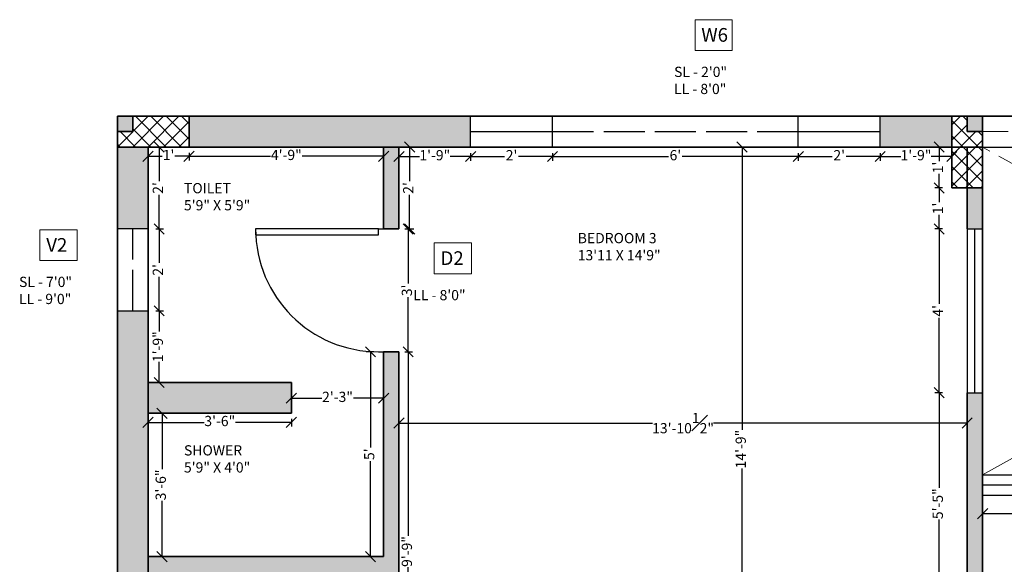
# Model space of a CAD drawing. Units: inches. Extents: x 1365 to 2091, y 1589 to 2091.
# Tile 4 of 8: x 1365 to 1654, y 1932 to 2091. Entities that reach past the tile are written whole.
import ezdxf

# ---------------------------------------------------------------- set-up
doc = ezdxf.new("R2010")
doc.units = ezdxf.units.IN
doc.linetypes.add('ACAD_ISO02W100', pattern=[15, 12, -3])
for name, color, linetype, lineweight in [('A-ANNO-DIMS', 2, 'Continuous', 18), ('A-ANNO-SYMB', 12, 'Continuous', 18), ('A-AREA-IDEN', 7, 'Continuous', 18), ('A-COLS', 7, 'Continuous', 35), ('A-COLS-MARK-PATT', 114, 'Continuous', 13), ('A-COLS-PATT', 1, 'Continuous', 13), ('A-DOOR', 4, 'Continuous', 25), ('A-FLOR-HRAL', 7, 'Continuous', 25), ('A-FLOR-OPEN', 7, 'Continuous', 25), ('A-FLOR-OPEN-HIDN', 1, 'ACAD_ISO02W100', 18), ('A-GLAZ', 150, 'Continuous', 30), ('A-GLAZ-HIDN', 150, 'ACAD_ISO02W100', 30), ('A-WALL', 7, 'Continuous', 35), ('A-WALL-PATT', 253, 'Continuous', 13)]:
    doc.layers.add(name, color=color, linetype=linetype, lineweight=lineweight)
doc.styles.get("Standard").update_dxf_attribs({"font": 'arial.ttf'})
doc.dimstyles.new('ISO-25', dxfattribs={"dimtxt": 3, "dimasz": 3, "dimexe": 1.25, "dimexo": 0.625, "dimtad": 0, "dimlunit": 4, "dimtxsty": 'Standard', "dimblk": 'OBLIQUE', "dimcen": 2.5, "dimclrd": 254, "dimclre": 254, "dimclrt": 1, "dimadec": 0, "dimazin": 0, "dimtfac": 1, "dimtmove": 0, "dimatfit": 3, "dimfxl": 1, "dimfxlon": 1, "dimfrac": 1, "dimarcsym": 0})

# ---------------------------------------------------------------- blocks, each defined once
blk = doc.blocks.new('*U3')
for p, q in [((-36, 0), (-36, -6)), ((0, 0), (0, -6))]:
    blk.add_line(p, q)
blk.add_lwpolyline([(0, 0), (0, 36), (-1.75, 36), (-1.75, 0)], close=True)
blk.add_arc((0, 0), 36, 90, 180)
blk = doc.blocks.new('_Oblique')
at = {"color": 0, "linetype": 'ByBlock', "lineweight": -2}
blk.add_line((-0.5, -0.5), (0.5, 0.5), dxfattribs=at)
blk = doc.blocks.new('*D8')
at = {"layer": 'A-ANNO-DIMS', "color": 0, "lineweight": -2, "transparency": 16777216}
for p, q in [((1402.75, 2052.14), (1402.75, 2049.89)), ((1414.75, 2052.14), (1414.75, 2049.89)), ((1402.75, 2051.14), (1406.89, 2051.14)), ((1414.75, 2051.14), (1410.62, 2051.14))]:
    blk.add_line(p, q, dxfattribs=at)
at = {"layer": 'Defpoints', "color": 0, "transparency": 16777216}
for p in [(1402.75, 2053.86), (1414.75, 2053.86), (1414.75, 2051.14)]:
    blk.add_point(p, dxfattribs=at)
at = {"layer": 'A-ANNO-DIMS', "color": 0, "lineweight": -2, "transparency": 16777216, "xscale": 3, "yscale": 3, "zscale": 3, "rotation": 180}
blk.add_blockref('_Oblique', (1402.75, 2051.14), dxfattribs=at)
at = {"layer": 'A-ANNO-DIMS', "color": 0, "lineweight": -2, "transparency": 16777216, "xscale": 3, "yscale": 3, "zscale": 3}
blk.add_blockref('_Oblique', (1414.75, 2051.14), dxfattribs=at)
at = {"layer": 'A-ANNO-DIMS', "color": 0, "transparency": 16777216, "insert": (1408.75, 2051.14), "char_height": 3, "attachment_point": 5}
blk.add_mtext("1'", dxfattribs=at)
blk = doc.blocks.new('*D9')
at = {"layer": 'A-ANNO-DIMS', "color": 0, "lineweight": -2, "transparency": 16777216}
for p, q in [((1414.75, 2052.14), (1414.75, 2049.89)), ((1471.75, 2052.14), (1471.75, 2049.89)), ((1414.75, 2051.14), (1438.58, 2051.14)), ((1471.75, 2051.14), (1447.93, 2051.14))]:
    blk.add_line(p, q, dxfattribs=at)
at = {"layer": 'Defpoints', "color": 0, "transparency": 16777216}
for p in [(1414.75, 2053.86), (1471.75, 2053.86), (1471.75, 2051.14)]:
    blk.add_point(p, dxfattribs=at)
at = {"layer": 'A-ANNO-DIMS', "color": 0, "lineweight": -2, "transparency": 16777216, "xscale": 3, "yscale": 3, "zscale": 3, "rotation": 180}
blk.add_blockref('_Oblique', (1414.75, 2051.14), dxfattribs=at)
at = {"layer": 'A-ANNO-DIMS', "color": 0, "lineweight": -2, "transparency": 16777216, "xscale": 3, "yscale": 3, "zscale": 3}
blk.add_blockref('_Oblique', (1471.75, 2051.14), dxfattribs=at)
at = {"layer": 'A-ANNO-DIMS', "color": 0, "transparency": 16777216, "insert": (1443.25, 2051.14), "char_height": 3, "attachment_point": 5}
blk.add_mtext('4\'-9"', dxfattribs=at)
blk = doc.blocks.new('*D10')
at = {"layer": 'A-ANNO-DIMS', "color": 0, "lineweight": -2, "transparency": 16777216}
for p, q in [((1476.25, 2052.07), (1476.25, 2049.82)), ((1497.25, 2052.07), (1497.25, 2049.82)), ((1476.25, 2051.07), (1482.28, 2051.07)), ((1497.25, 2051.07), (1491.22, 2051.07))]:
    blk.add_line(p, q, dxfattribs=at)
at = {"layer": 'Defpoints', "color": 0, "transparency": 16777216}
for p in [(1476.25, 2053.86), (1497.25, 2053.86), (1476.25, 2051.07)]:
    blk.add_point(p, dxfattribs=at)
at = {"layer": 'A-ANNO-DIMS', "color": 0, "lineweight": -2, "transparency": 16777216, "xscale": 3, "yscale": 3, "zscale": 3, "rotation": 180}
blk.add_blockref('_Oblique', (1476.25, 2051.07), dxfattribs=at)
at = {"layer": 'A-ANNO-DIMS', "color": 0, "lineweight": -2, "transparency": 16777216, "xscale": 3, "yscale": 3, "zscale": 3}
blk.add_blockref('_Oblique', (1497.25, 2051.07), dxfattribs=at)
at = {"layer": 'A-ANNO-DIMS', "color": 0, "transparency": 16777216, "insert": (1486.75, 2051.07), "char_height": 3, "attachment_point": 5}
blk.add_mtext('1\'-9"', dxfattribs=at)
blk = doc.blocks.new('*D11')
at = {"layer": 'A-ANNO-DIMS', "color": 0, "lineweight": -2, "transparency": 16777216}
for p, q in [((1497.25, 2052.07), (1497.25, 2049.82)), ((1521.25, 2052.07), (1521.25, 2049.82)), ((1497.25, 2051.07), (1507.22, 2051.07)), ((1521.25, 2051.07), (1511.28, 2051.07))]:
    blk.add_line(p, q, dxfattribs=at)
at = {"layer": 'Defpoints', "color": 0, "transparency": 16777216}
for p in [(1497.25, 2053.86), (1521.25, 2053.86), (1521.25, 2051.07)]:
    blk.add_point(p, dxfattribs=at)
at = {"layer": 'A-ANNO-DIMS', "color": 0, "lineweight": -2, "transparency": 16777216, "xscale": 3, "yscale": 3, "zscale": 3, "rotation": 180}
blk.add_blockref('_Oblique', (1497.25, 2051.07), dxfattribs=at)
at = {"layer": 'A-ANNO-DIMS', "color": 0, "lineweight": -2, "transparency": 16777216, "xscale": 3, "yscale": 3, "zscale": 3}
blk.add_blockref('_Oblique', (1521.25, 2051.07), dxfattribs=at)
at = {"layer": 'A-ANNO-DIMS', "color": 0, "transparency": 16777216, "insert": (1509.25, 2051.07), "char_height": 3, "attachment_point": 5}
blk.add_mtext("2'", dxfattribs=at)
blk = doc.blocks.new('*D12')
at = {"layer": 'A-ANNO-DIMS', "color": 0, "lineweight": -2, "transparency": 16777216}
for p, q in [((1521.25, 2052.07), (1521.25, 2049.82)), ((1593.25, 2052.07), (1593.25, 2049.82)), ((1521.25, 2051.07), (1555.24, 2051.07)), ((1593.25, 2051.07), (1559.27, 2051.07))]:
    blk.add_line(p, q, dxfattribs=at)
at = {"layer": 'Defpoints', "color": 0, "transparency": 16777216}
for p in [(1521.25, 2053.86), (1593.25, 2053.86), (1593.25, 2051.07)]:
    blk.add_point(p, dxfattribs=at)
at = {"layer": 'A-ANNO-DIMS', "color": 0, "lineweight": -2, "transparency": 16777216, "xscale": 3, "yscale": 3, "zscale": 3, "rotation": 180}
blk.add_blockref('_Oblique', (1521.25, 2051.07), dxfattribs=at)
at = {"layer": 'A-ANNO-DIMS', "color": 0, "lineweight": -2, "transparency": 16777216, "xscale": 3, "yscale": 3, "zscale": 3}
blk.add_blockref('_Oblique', (1593.25, 2051.07), dxfattribs=at)
at = {"layer": 'A-ANNO-DIMS', "color": 0, "transparency": 16777216, "insert": (1557.25, 2051.07), "char_height": 3, "attachment_point": 5}
blk.add_mtext("6'", dxfattribs=at)
blk = doc.blocks.new('*D13')
at = {"layer": 'A-ANNO-DIMS', "color": 0, "lineweight": -2, "transparency": 16777216}
for p, q in [((1593.25, 2052.07), (1593.25, 2049.82)), ((1617.25, 2052.07), (1617.25, 2049.82)), ((1593.25, 2051.07), (1603.22, 2051.07)), ((1617.25, 2051.07), (1607.28, 2051.07))]:
    blk.add_line(p, q, dxfattribs=at)
at = {"layer": 'Defpoints', "color": 0, "transparency": 16777216}
for p in [(1593.25, 2053.86), (1617.25, 2053.86), (1617.25, 2051.07)]:
    blk.add_point(p, dxfattribs=at)
at = {"layer": 'A-ANNO-DIMS', "color": 0, "lineweight": -2, "transparency": 16777216, "xscale": 3, "yscale": 3, "zscale": 3, "rotation": 180}
blk.add_blockref('_Oblique', (1593.25, 2051.07), dxfattribs=at)
at = {"layer": 'A-ANNO-DIMS', "color": 0, "lineweight": -2, "transparency": 16777216, "xscale": 3, "yscale": 3, "zscale": 3}
blk.add_blockref('_Oblique', (1617.25, 2051.07), dxfattribs=at)
at = {"layer": 'A-ANNO-DIMS', "color": 0, "transparency": 16777216, "insert": (1605.25, 2051.07), "char_height": 3, "attachment_point": 5}
blk.add_mtext("2'", dxfattribs=at)
blk = doc.blocks.new('*D14')
at = {"layer": 'A-ANNO-DIMS', "color": 0, "lineweight": -2, "transparency": 16777216}
for p, q in [((1617.25, 2052.07), (1617.25, 2049.82)), ((1638.25, 2052.07), (1638.25, 2049.82)), ((1617.25, 2051.07), (1623.28, 2051.07)), ((1638.25, 2051.07), (1632.22, 2051.07))]:
    blk.add_line(p, q, dxfattribs=at)
at = {"layer": 'Defpoints', "color": 0, "transparency": 16777216}
for p in [(1617.25, 2053.86), (1638.25, 2053.86), (1638.25, 2051.07)]:
    blk.add_point(p, dxfattribs=at)
at = {"layer": 'A-ANNO-DIMS', "color": 0, "lineweight": -2, "transparency": 16777216, "xscale": 3, "yscale": 3, "zscale": 3, "rotation": 180}
blk.add_blockref('_Oblique', (1617.25, 2051.07), dxfattribs=at)
at = {"layer": 'A-ANNO-DIMS', "color": 0, "lineweight": -2, "transparency": 16777216, "xscale": 3, "yscale": 3, "zscale": 3}
blk.add_blockref('_Oblique', (1638.25, 2051.07), dxfattribs=at)
at = {"layer": 'A-ANNO-DIMS', "color": 0, "transparency": 16777216, "insert": (1627.75, 2051.07), "char_height": 3, "attachment_point": 5}
blk.add_mtext('1\'-9"', dxfattribs=at)
blk = doc.blocks.new('*D16')
at = {"layer": 'A-ANNO-DIMS', "color": 0, "lineweight": -2, "transparency": 16777216}
for p, q in [((1404.99, 2053.86), (1407.24, 2053.86)), ((1405.99, 2053.86), (1405.99, 2043.89)), ((1405.99, 2029.86), (1405.99, 2039.83)), ((1404.99, 2029.86), (1407.24, 2029.86))]:
    blk.add_line(p, q, dxfattribs=at)
at = {"layer": 'Defpoints', "color": 0, "transparency": 16777216}
for p in [(1402.75, 2053.86), (1402.75, 2029.86), (1405.99, 2029.86)]:
    blk.add_point(p, dxfattribs=at)
at = {"layer": 'A-ANNO-DIMS', "color": 0, "lineweight": -2, "transparency": 16777216, "xscale": 3, "yscale": 3, "zscale": 3}
for p, rotation in [((1405.99, 2053.86), 90), ((1405.99, 2029.86), 270)]:
    blk.add_blockref('_Oblique', p, dxfattribs=dict(at, rotation=rotation))
at = {"layer": 'A-ANNO-DIMS', "color": 0, "transparency": 16777216, "insert": (1405.99, 2041.86), "char_height": 3, "attachment_point": 5, "rotation": 90}
blk.add_mtext("2'", dxfattribs=at)
blk = doc.blocks.new('*D17')
at = {"layer": 'A-ANNO-DIMS', "color": 0, "lineweight": -2, "transparency": 16777216}
for p, q in [((1404.99, 2029.86), (1407.24, 2029.86)), ((1405.99, 2029.86), (1405.99, 2019.89)), ((1405.99, 2005.86), (1405.99, 2015.83)), ((1404.99, 2005.86), (1407.24, 2005.86))]:
    blk.add_line(p, q, dxfattribs=at)
at = {"layer": 'Defpoints', "color": 0, "transparency": 16777216}
for p in [(1402.75, 2029.86), (1402.75, 2005.86), (1405.99, 2005.86)]:
    blk.add_point(p, dxfattribs=at)
at = {"layer": 'A-ANNO-DIMS', "color": 0, "lineweight": -2, "transparency": 16777216, "xscale": 3, "yscale": 3, "zscale": 3}
for p, rotation in [((1405.99, 2029.86), 90), ((1405.99, 2005.86), 270)]:
    blk.add_blockref('_Oblique', p, dxfattribs=dict(at, rotation=rotation))
at = {"layer": 'A-ANNO-DIMS', "color": 0, "transparency": 16777216, "insert": (1405.99, 2017.86), "char_height": 3, "attachment_point": 5, "rotation": 90}
blk.add_mtext("2'", dxfattribs=at)
blk = doc.blocks.new('*D18')
at = {"layer": 'A-ANNO-DIMS', "color": 0, "lineweight": -2, "transparency": 16777216}
for p, q in [((1404.99, 2005.86), (1407.24, 2005.86)), ((1405.99, 2005.86), (1405.99, 1999.83)), ((1405.99, 1984.86), (1405.99, 1990.89)), ((1404.99, 1984.86), (1407.24, 1984.86))]:
    blk.add_line(p, q, dxfattribs=at)
at = {"layer": 'Defpoints', "color": 0, "transparency": 16777216}
for p in [(1402.75, 2005.86), (1402.75, 1984.86), (1405.99, 1984.86)]:
    blk.add_point(p, dxfattribs=at)
at = {"layer": 'A-ANNO-DIMS', "color": 0, "lineweight": -2, "transparency": 16777216, "xscale": 3, "yscale": 3, "zscale": 3}
for p, rotation in [((1405.99, 2005.86), 90), ((1405.99, 1984.86), 270)]:
    blk.add_blockref('_Oblique', p, dxfattribs=dict(at, rotation=rotation))
at = {"layer": 'A-ANNO-DIMS', "color": 0, "transparency": 16777216, "insert": (1405.99, 1995.36), "char_height": 3, "attachment_point": 5, "rotation": 90}
blk.add_mtext('1\'-9"', dxfattribs=at)
blk = doc.blocks.new('*D19')
at = {"layer": 'A-ANNO-DIMS', "color": 0, "lineweight": -2, "transparency": 16777216}
for p, q in [((1444.75, 1979.27), (1444.75, 1981.52)), ((1444.75, 1980.27), (1453.62, 1980.27)), ((1471.75, 1980.27), (1462.89, 1980.27)), ((1471.75, 1979.27), (1471.75, 1981.52))]:
    blk.add_line(p, q, dxfattribs=at)
at = {"layer": 'Defpoints', "color": 0, "transparency": 16777216}
for p in [(1471.75, 1980.27), (1444.75, 1975.86), (1471.75, 1975.86)]:
    blk.add_point(p, dxfattribs=at)
at = {"layer": 'A-ANNO-DIMS', "color": 0, "lineweight": -2, "transparency": 16777216, "xscale": 3, "yscale": 3, "zscale": 3, "rotation": 180}
blk.add_blockref('_Oblique', (1444.75, 1980.27), dxfattribs=at)
at = {"layer": 'A-ANNO-DIMS', "color": 0, "lineweight": -2, "transparency": 16777216, "xscale": 3, "yscale": 3, "zscale": 3}
blk.add_blockref('_Oblique', (1471.75, 1980.27), dxfattribs=at)
at = {"layer": 'A-ANNO-DIMS', "color": 0, "transparency": 16777216, "insert": (1458.25, 1980.27), "char_height": 3, "attachment_point": 5}
blk.add_mtext('2\'-3"', dxfattribs=at)
blk = doc.blocks.new('*D20')
at = {"layer": 'A-ANNO-DIMS', "color": 0, "lineweight": -2, "transparency": 16777216}
for p, q in [((1402.75, 1974.2), (1402.75, 1971.95)), ((1444.75, 1974.2), (1444.75, 1971.95)), ((1402.75, 1973.2), (1419.14, 1973.2)), ((1444.75, 1973.2), (1428.37, 1973.2))]:
    blk.add_line(p, q, dxfattribs=at)
at = {"layer": 'Defpoints', "color": 0, "transparency": 16777216}
for p in [(1402.75, 1975.86), (1444.75, 1975.86), (1444.75, 1973.2)]:
    blk.add_point(p, dxfattribs=at)
at = {"layer": 'A-ANNO-DIMS', "color": 0, "lineweight": -2, "transparency": 16777216, "xscale": 3, "yscale": 3, "zscale": 3, "rotation": 180}
blk.add_blockref('_Oblique', (1402.75, 1973.2), dxfattribs=at)
at = {"layer": 'A-ANNO-DIMS', "color": 0, "lineweight": -2, "transparency": 16777216, "xscale": 3, "yscale": 3, "zscale": 3}
blk.add_blockref('_Oblique', (1444.75, 1973.2), dxfattribs=at)
at = {"layer": 'A-ANNO-DIMS', "color": 0, "transparency": 16777216, "insert": (1423.75, 1973.2), "char_height": 3, "attachment_point": 5}
blk.add_mtext('3\'-6"', dxfattribs=at)
blk = doc.blocks.new('*D21')
at = {"layer": 'A-ANNO-DIMS', "color": 0, "lineweight": -2, "transparency": 16777216}
for p, q in [((1405.84, 1975.86), (1408.09, 1975.86)), ((1406.84, 1975.86), (1406.84, 1959.47)), ((1406.84, 1933.86), (1406.84, 1950.25)), ((1405.84, 1933.86), (1408.09, 1933.86))]:
    blk.add_line(p, q, dxfattribs=at)
at = {"layer": 'Defpoints', "color": 0, "transparency": 16777216}
for p in [(1402.75, 1975.86), (1406.84, 1975.86), (1402.75, 1933.86)]:
    blk.add_point(p, dxfattribs=at)
at = {"layer": 'A-ANNO-DIMS', "color": 0, "lineweight": -2, "transparency": 16777216, "xscale": 3, "yscale": 3, "zscale": 3}
for p, rotation in [((1406.84, 1975.86), 90), ((1406.84, 1933.86), 270)]:
    blk.add_blockref('_Oblique', p, dxfattribs=dict(at, rotation=rotation))
at = {"layer": 'A-ANNO-DIMS', "color": 0, "transparency": 16777216, "insert": (1406.84, 1954.86), "char_height": 3, "attachment_point": 5, "rotation": 90}
blk.add_mtext('3\'-6"', dxfattribs=at)
blk = doc.blocks.new('*D22')
at = {"layer": 'A-ANNO-DIMS', "color": 0, "lineweight": -2, "transparency": 16777216}
for p, q in [((1468.92, 1993.86), (1466.67, 1993.86)), ((1467.92, 1993.86), (1467.92, 1965.86)), ((1467.92, 1933.86), (1467.92, 1961.85)), ((1468.92, 1933.86), (1466.67, 1933.86))]:
    blk.add_line(p, q, dxfattribs=at)
at = {"layer": 'Defpoints', "color": 0, "transparency": 16777216}
for p in [(1471.75, 1993.86), (1467.92, 1933.86), (1471.75, 1933.86)]:
    blk.add_point(p, dxfattribs=at)
at = {"layer": 'A-ANNO-DIMS', "color": 0, "lineweight": -2, "transparency": 16777216, "xscale": 3, "yscale": 3, "zscale": 3}
for p, rotation in [((1467.92, 1993.86), 90), ((1467.92, 1933.86), 270)]:
    blk.add_blockref('_Oblique', p, dxfattribs=dict(at, rotation=rotation))
at = {"layer": 'A-ANNO-DIMS', "color": 0, "transparency": 16777216, "insert": (1467.92, 1963.86), "char_height": 3, "attachment_point": 5, "rotation": 90}
blk.add_mtext("5'", dxfattribs=at)
blk = doc.blocks.new('*D93')
at = {"layer": 'A-ANNO-DIMS', "color": 0, "lineweight": -2, "transparency": 16777216}
for p, q in [((1647.25, 1947.47), (1647.25, 1945.22)), ((1819.75, 1947.47), (1819.75, 1945.22)), ((1647.25, 1946.47), (1725.72, 1946.47)), ((1819.75, 1946.47), (1741.29, 1946.47))]:
    blk.add_line(p, q, dxfattribs=at)
at = {"layer": 'Defpoints', "color": 0, "transparency": 16777216}
for p in [(1647.25, 1951.86), (1819.75, 1951.86), (1819.75, 1946.47)]:
    blk.add_point(p, dxfattribs=at)
at = {"layer": 'A-ANNO-DIMS', "color": 0, "lineweight": -2, "transparency": 16777216, "xscale": 3, "yscale": 3, "zscale": 3, "rotation": 180}
blk.add_blockref('_Oblique', (1647.25, 1946.47), dxfattribs=at)
at = {"layer": 'A-ANNO-DIMS', "color": 0, "lineweight": -2, "transparency": 16777216, "xscale": 3, "yscale": 3, "zscale": 3}
blk.add_blockref('_Oblique', (1819.75, 1946.47), dxfattribs=at)
at = {"layer": 'A-ANNO-DIMS', "color": 0, "transparency": 16777216, "insert": (1733.5, 1946.47), "char_height": 3, "attachment_point": 5}
blk.add_mtext('14\'-4{\\H1x;\\S1#2;}"', dxfattribs=at)
blk = doc.blocks.new('*D94')
at = {"layer": 'A-ANNO-DIMS', "color": 0, "lineweight": -2, "transparency": 16777216}
for p, q in [((1635.53, 2053.86), (1633.28, 2053.86)), ((1634.53, 2053.86), (1634.53, 2049.72)), ((1634.53, 2041.86), (1634.53, 2045.99)), ((1635.53, 2041.86), (1633.28, 2041.86))]:
    blk.add_line(p, q, dxfattribs=at)
at = {"layer": 'Defpoints', "color": 0, "transparency": 16777216}
for p in [(1638.25, 2053.86), (1634.53, 2041.86), (1638.25, 2041.86)]:
    blk.add_point(p, dxfattribs=at)
at = {"layer": 'A-ANNO-DIMS', "color": 0, "lineweight": -2, "transparency": 16777216, "xscale": 3, "yscale": 3, "zscale": 3}
for p, rotation in [((1634.53, 2053.86), 90), ((1634.53, 2041.86), 270)]:
    blk.add_blockref('_Oblique', p, dxfattribs=dict(at, rotation=rotation))
at = {"layer": 'A-ANNO-DIMS', "color": 0, "transparency": 16777216, "insert": (1634.53, 2047.86), "char_height": 3, "attachment_point": 5, "rotation": 90}
blk.add_mtext("1'", dxfattribs=at)
blk = doc.blocks.new('*D95')
at = {"layer": 'A-ANNO-DIMS', "color": 0, "lineweight": -2, "transparency": 16777216}
for p, q in [((1635.53, 2041.86), (1633.28, 2041.86)), ((1634.53, 2041.86), (1634.53, 2037.72)), ((1634.53, 2029.86), (1634.53, 2033.99)), ((1635.53, 2029.86), (1633.28, 2029.86))]:
    blk.add_line(p, q, dxfattribs=at)
at = {"layer": 'Defpoints', "color": 0, "transparency": 16777216}
for p in [(1638.25, 2041.86), (1634.53, 2029.86), (1642.75, 2029.86)]:
    blk.add_point(p, dxfattribs=at)
at = {"layer": 'A-ANNO-DIMS', "color": 0, "lineweight": -2, "transparency": 16777216, "xscale": 3, "yscale": 3, "zscale": 3}
for p, rotation in [((1634.53, 2041.86), 90), ((1634.53, 2029.86), 270)]:
    blk.add_blockref('_Oblique', p, dxfattribs=dict(at, rotation=rotation))
at = {"layer": 'A-ANNO-DIMS', "color": 0, "transparency": 16777216, "insert": (1634.53, 2035.86), "char_height": 3, "attachment_point": 5, "rotation": 90}
blk.add_mtext("1'", dxfattribs=at)
blk = doc.blocks.new('*D96')
at = {"layer": 'A-ANNO-DIMS', "color": 0, "lineweight": -2, "transparency": 16777216}
for p, q in [((1635.53, 2029.86), (1633.28, 2029.86)), ((1634.53, 2029.86), (1634.53, 2007.92)), ((1634.53, 1981.86), (1634.53, 2003.79)), ((1635.53, 1981.86), (1633.28, 1981.86))]:
    blk.add_line(p, q, dxfattribs=at)
at = {"layer": 'Defpoints', "color": 0, "transparency": 16777216}
for p in [(1642.75, 2029.86), (1634.53, 1981.86), (1642.75, 1981.86)]:
    blk.add_point(p, dxfattribs=at)
at = {"layer": 'A-ANNO-DIMS', "color": 0, "lineweight": -2, "transparency": 16777216, "xscale": 3, "yscale": 3, "zscale": 3}
for p, rotation in [((1634.53, 2029.86), 90), ((1634.53, 1981.86), 270)]:
    blk.add_blockref('_Oblique', p, dxfattribs=dict(at, rotation=rotation))
at = {"layer": 'A-ANNO-DIMS', "color": 0, "transparency": 16777216, "insert": (1634.53, 2005.86), "char_height": 3, "attachment_point": 5, "rotation": 90}
blk.add_mtext("4'", dxfattribs=at)
blk = doc.blocks.new('*D97')
at = {"layer": 'A-ANNO-DIMS', "color": 0, "lineweight": -2, "transparency": 16777216}
for p, q in [((1635.53, 1981.86), (1633.28, 1981.86)), ((1634.53, 1981.86), (1634.53, 1953.97)), ((1634.53, 1916.86), (1634.53, 1944.75)), ((1635.53, 1916.86), (1633.28, 1916.86))]:
    blk.add_line(p, q, dxfattribs=at)
at = {"layer": 'Defpoints', "color": 0, "transparency": 16777216}
for p in [(1642.75, 1981.86), (1634.53, 1916.86), (1642.75, 1916.86)]:
    blk.add_point(p, dxfattribs=at)
at = {"layer": 'A-ANNO-DIMS', "color": 0, "lineweight": -2, "transparency": 16777216, "xscale": 3, "yscale": 3, "zscale": 3}
for p, rotation in [((1634.53, 1981.86), 90), ((1634.53, 1916.86), 270)]:
    blk.add_blockref('_Oblique', p, dxfattribs=dict(at, rotation=rotation))
at = {"layer": 'A-ANNO-DIMS', "color": 0, "transparency": 16777216, "insert": (1634.53, 1949.36), "char_height": 3, "attachment_point": 5, "rotation": 90}
blk.add_mtext('5\'-5"', dxfattribs=at)
blk = doc.blocks.new('*D110')
at = {"layer": 'A-ANNO-DIMS', "color": 0, "lineweight": -2, "transparency": 16777216}
for p, q in [((1478.36, 2053.86), (1480.61, 2053.86)), ((1479.36, 2053.86), (1479.36, 2043.89)), ((1479.36, 2029.86), (1479.36, 2039.83)), ((1478.36, 2029.86), (1480.61, 2029.86))]:
    blk.add_line(p, q, dxfattribs=at)
at = {"layer": 'Defpoints', "color": 0, "transparency": 16777216}
for p in [(1476.25, 2053.86), (1479.36, 2053.86), (1476.25, 2029.86)]:
    blk.add_point(p, dxfattribs=at)
at = {"layer": 'A-ANNO-DIMS', "color": 0, "lineweight": -2, "transparency": 16777216, "xscale": 3, "yscale": 3, "zscale": 3}
for p, rotation in [((1479.36, 2053.86), 90), ((1479.36, 2029.86), 270)]:
    blk.add_blockref('_Oblique', p, dxfattribs=dict(at, rotation=rotation))
at = {"layer": 'A-ANNO-DIMS', "color": 0, "transparency": 16777216, "insert": (1479.36, 2041.86), "char_height": 3, "attachment_point": 5, "rotation": 90}
blk.add_mtext("2'", dxfattribs=at)
blk = doc.blocks.new('*D111')
at = {"layer": 'A-ANNO-DIMS', "color": 0, "lineweight": -2, "transparency": 16777216}
for p, q in [((1477.96, 2029.86), (1480.21, 2029.86)), ((1478.96, 2029.86), (1478.96, 2013.86)), ((1478.96, 1993.86), (1478.96, 2009.85)), ((1477.96, 1993.86), (1480.21, 1993.86))]:
    blk.add_line(p, q, dxfattribs=at)
at = {"layer": 'Defpoints', "color": 0, "transparency": 16777216}
for p in [(1476.25, 2029.86), (1476.25, 1993.86), (1478.96, 1993.86)]:
    blk.add_point(p, dxfattribs=at)
at = {"layer": 'A-ANNO-DIMS', "color": 0, "lineweight": -2, "transparency": 16777216, "xscale": 3, "yscale": 3, "zscale": 3}
for p, rotation in [((1478.96, 2029.86), 90), ((1478.96, 1993.86), 270)]:
    blk.add_blockref('_Oblique', p, dxfattribs=dict(at, rotation=rotation))
at = {"layer": 'A-ANNO-DIMS', "color": 0, "transparency": 16777216, "insert": (1478.96, 2011.86), "char_height": 3, "attachment_point": 5, "rotation": 90}
blk.add_mtext("3'", dxfattribs=at)
blk = doc.blocks.new('*D112')
at = {"layer": 'A-ANNO-DIMS', "color": 0, "lineweight": -2, "transparency": 16777216}
for p, q in [((1477.96, 1993.86), (1480.21, 1993.86)), ((1478.96, 1993.86), (1478.96, 1939.97)), ((1478.96, 1876.86), (1478.96, 1930.75)), ((1477.96, 1876.86), (1480.21, 1876.86))]:
    blk.add_line(p, q, dxfattribs=at)
at = {"layer": 'Defpoints', "color": 0, "transparency": 16777216}
for p in [(1476.25, 1993.86), (1476.25, 1876.86), (1478.96, 1876.86)]:
    blk.add_point(p, dxfattribs=at)
at = {"layer": 'A-ANNO-DIMS', "color": 0, "lineweight": -2, "transparency": 16777216, "xscale": 3, "yscale": 3, "zscale": 3}
for p, rotation in [((1478.96, 1993.86), 90), ((1478.96, 1876.86), 270)]:
    blk.add_blockref('_Oblique', p, dxfattribs=dict(at, rotation=rotation))
at = {"layer": 'A-ANNO-DIMS', "color": 0, "transparency": 16777216, "insert": (1478.96, 1935.36), "char_height": 3, "attachment_point": 5, "rotation": 90}
blk.add_mtext('9\'-9"', dxfattribs=at)
blk = doc.blocks.new('*D115')
at = {"layer": 'A-ANNO-DIMS', "color": 0, "lineweight": -2, "transparency": 16777216}
for p, q in [((1476.25, 1973.98), (1476.25, 1971.73)), ((1642.75, 1973.98), (1642.75, 1971.73)), ((1476.25, 1972.98), (1550.56, 1972.98)), ((1642.75, 1972.98), (1568.45, 1972.98))]:
    blk.add_line(p, q, dxfattribs=at)
at = {"layer": 'Defpoints', "color": 0, "transparency": 16777216}
for p in [(1476.25, 1993.86), (1642.75, 1993.86), (1642.75, 1972.98)]:
    blk.add_point(p, dxfattribs=at)
at = {"layer": 'A-ANNO-DIMS', "color": 0, "lineweight": -2, "transparency": 16777216, "xscale": 3, "yscale": 3, "zscale": 3, "rotation": 180}
blk.add_blockref('_Oblique', (1476.25, 1972.98), dxfattribs=at)
at = {"layer": 'A-ANNO-DIMS', "color": 0, "lineweight": -2, "transparency": 16777216, "xscale": 3, "yscale": 3, "zscale": 3}
blk.add_blockref('_Oblique', (1642.75, 1972.98), dxfattribs=at)
at = {"layer": 'A-ANNO-DIMS', "color": 0, "transparency": 16777216, "insert": (1559.5, 1972.98), "char_height": 3, "attachment_point": 5}
blk.add_mtext('13\'-10{\\H1x;\\S1#2;}"', dxfattribs=at)
blk = doc.blocks.new('*D116')
at = {"layer": 'A-ANNO-DIMS', "color": 0, "lineweight": -2, "transparency": 16777216}
for p, q in [((1575.79, 2053.86), (1578.04, 2053.86)), ((1576.79, 2053.86), (1576.79, 1970.99)), ((1576.79, 1876.86), (1576.79, 1959.72)), ((1575.79, 1876.86), (1578.04, 1876.86))]:
    blk.add_line(p, q, dxfattribs=at)
at = {"layer": 'Defpoints', "color": 0, "transparency": 16777216}
for p in [(1550.15, 2053.86), (1550.15, 1876.86), (1576.79, 1876.86)]:
    blk.add_point(p, dxfattribs=at)
at = {"layer": 'A-ANNO-DIMS', "color": 0, "lineweight": -2, "transparency": 16777216, "xscale": 3, "yscale": 3, "zscale": 3}
for p, rotation in [((1576.79, 2053.86), 90), ((1576.79, 1876.86), 270)]:
    blk.add_blockref('_Oblique', p, dxfattribs=dict(at, rotation=rotation))
at = {"layer": 'A-ANNO-DIMS', "color": 0, "transparency": 16777216, "insert": (1576.79, 1965.36), "char_height": 3, "attachment_point": 5, "rotation": 90}
blk.add_mtext('14\'-9"', dxfattribs=at)
blk = doc.blocks.new('OPENING-TAG-V2')
blk.add_lwpolyline([(6.13, 13.79), (17.02, 13.79), (17.02, 4.75), (6.13, 4.75)], close=True)
at = {"attachment_point": 1}
for s, width, insert, char_height in [('{V2}', 14.5136, (7.98, 11.34), 4), ('{SL - 7\'0"\\PLL - 9\'0"}', 24.3857, (0, 0), 3)]:
    blk.add_mtext_dynamic_manual_height_columns(s, width=width, gutter_width=12.5, heights=[0], dxfattribs=dict(at, insert=insert, char_height=char_height))
blk = doc.blocks.new('OPENING-TAG-D2')
blk.add_lwpolyline([(6.13, 13.79), (17.02, 13.79), (17.02, 4.75), (6.13, 4.75)], close=True)
at = {"attachment_point": 1}
for s, width, insert, char_height in [('{D2}', 14.5136, (7.98, 11.34), 4), ('{LL - 8\'0"}', 24.3857, (0, 0), 3)]:
    blk.add_mtext_dynamic_manual_height_columns(s, width=width, gutter_width=12.5, heights=[0], dxfattribs=dict(at, insert=insert, char_height=char_height))

msp = doc.modelspace()

# ---------------------------------------------------------------- hatches: boundary and pattern name
at = {"layer": 'A-COLS-MARK-PATT'}
h = msp.add_hatch(color=256, dxfattribs=at)
h.dxf.hatch_style = 1
h.paths.add_polyline_path([(1398.254, 2062.858), (1393.754, 2062.858), (1393.754, 2058.358), (1398.254, 2058.358)])
h.paths.add_polyline_path([(1398.254, 1872.358), (1393.754, 1872.358), (1393.754, 1867.858), (1398.254, 1867.858)])
h.paths.add_polyline_path([(1398.254, 1807.858), (1393.754, 1807.858), (1393.754, 1803.358), (1398.254, 1803.358)])
h.paths.add_polyline_path([(1398.254, 1647.358), (1393.754, 1647.358), (1393.754, 1642.858), (1398.254, 1642.858)])
h.paths.add_polyline_path([(1638.254, 1647.358), (1633.754, 1647.358), (1633.754, 1642.858), (1638.254, 1642.858)])
h.paths.add_polyline_path([(1638.254, 1732.858), (1633.754, 1732.858), (1633.754, 1728.358), (1638.254, 1728.358)])
h.paths.add_polyline_path([(1647.254, 1876.858), (1642.754, 1876.858), (1642.754, 1872.358), (1647.254, 1872.358)])
h.paths.add_polyline_path([(1647.254, 1803.358), (1642.754, 1803.358), (1642.754, 1798.858), (1647.254, 1798.858)])
h.paths.add_polyline_path([(1647.254, 2062.858), (1642.754, 2062.858), (1642.754, 2058.358), (1647.254, 2058.358)])
h.paths.add_polyline_path([(1824.254, 2062.858), (1819.754, 2062.858), (1819.754, 2058.358), (1824.254, 2058.358)])
h.paths.add_polyline_path([(1824.254, 1885.858), (1819.754, 1885.858), (1819.754, 1881.358), (1824.254, 1881.358)])
h.paths.add_polyline_path([(1828.754, 1647.358), (1824.254, 1647.358), (1824.254, 1642.858), (1828.754, 1642.858)])
h.paths.add_polyline_path([(1948.754, 1647.358), (1944.254, 1647.358), (1944.254, 1642.858), (1948.754, 1642.858)])
h.paths.add_polyline_path([(2041.754, 1647.358), (2037.254, 1647.358), (2037.254, 1642.858), (2041.754, 1642.858)])
h.paths.add_polyline_path([(2041.754, 1885.858), (2037.254, 1885.858), (2037.254, 1881.358), (2041.754, 1881.358)])
h.paths.add_polyline_path([(2041.754, 2062.858), (2037.254, 2062.858), (2037.254, 2058.358), (2041.754, 2058.358)])
at = {"layer": 'A-COLS-PATT'}
h = msp.add_hatch(dxfattribs=at)
h.set_pattern_fill('ANSI37', color=256)
h.paths.add_polyline_path([(1414.754, 2062.858), (1398.254, 2062.858), (1398.254, 2058.358), (1393.754, 2058.358), (1393.754, 2053.858), (1414.754, 2053.858)])
h.paths.add_polyline_path([(1402.754, 1888.858), (1393.754, 1888.858), (1393.754, 1872.358), (1398.254, 1872.358), (1398.254, 1867.858), (1402.754, 1867.858), (1402.754, 1872.358)])
h.paths.add_polyline_path([(1402.754, 1807.858), (1398.254, 1807.858), (1398.254, 1803.358), (1393.754, 1803.358), (1393.754, 1789.858), (1402.754, 1789.858)])
h.paths.add_polyline_path([(1402.754, 1663.858), (1393.754, 1663.858), (1393.754, 1647.358), (1398.254, 1647.358), (1398.254, 1642.858), (1402.754, 1642.858)])
h.paths.add_polyline_path([(1638.254, 1666.858), (1629.254, 1666.858), (1629.254, 1642.858), (1633.754, 1642.858), (1633.754, 1647.358), (1638.254, 1647.358)])
h.paths.add_polyline_path([(1633.754, 1732.858), (1629.254, 1732.858), (1629.254, 1714.858), (1633.754, 1714.858)])
h.paths.add_polyline_path([(1638.254, 1728.358), (1633.754, 1728.358), (1633.754, 1714.858), (1638.254, 1714.858)])
h = msp.add_hatch(dxfattribs=at)
h.set_pattern_fill('ANSI37', color=256)
h.paths.add_polyline_path([(1642.754, 1803.358), (1647.254, 1803.358), (1647.254, 1807.858), (1629.254, 1807.858), (1629.254, 1798.858), (1633.754, 1798.858), (1642.754, 1798.858)])
h.paths.add_polyline_path([(1647.254, 1872.358), (1642.754, 1872.358), (1642.754, 1876.858), (1641.254, 1876.858), (1623.254, 1876.858), (1623.254, 1867.858), (1638.254, 1867.858), (1647.254, 1867.858)])
h.paths.add_polyline_path([(1647.254, 2058.358), (1642.754, 2058.358), (1642.754, 2062.858), (1638.254, 2062.858), (1638.254, 2053.858), (1647.254, 2053.858)])
h.paths.add_polyline_path([(1642.754, 2053.858), (1638.254, 2053.858), (1638.254, 2041.858), (1642.754, 2041.858)])
h.paths.add_polyline_path([(1647.254, 2053.858), (1642.754, 2053.858), (1642.754, 2041.858), (1647.254, 2041.858)])
h.paths.add_polyline_path([(1828.754, 2062.858), (1824.254, 2062.858), (1824.254, 2058.358), (1819.754, 2058.358), (1819.754, 2038.858), (1828.754, 2038.858)])
h.paths.add_polyline_path([(1839.254, 1885.858), (1825.754, 1885.858), (1824.254, 1885.858), (1824.254, 1881.358), (1819.754, 1881.358), (1819.754, 1876.858), (1839.254, 1876.858)])
h.paths.add_polyline_path([(2041.754, 1881.358), (2037.254, 1881.358), (2037.254, 1885.858), (2023.754, 1885.858), (2023.754, 1876.858), (2041.754, 1876.858)])
h.paths.add_polyline_path([(1828.754, 1666.858), (1819.754, 1666.858), (1819.754, 1642.858), (1824.254, 1642.858), (1824.254, 1647.358), (1828.754, 1647.358)])
h.paths.add_polyline_path([(1944.254, 1647.358), (1948.754, 1647.358), (1948.754, 1651.858), (1930.754, 1651.858), (1930.754, 1642.858), (1944.254, 1642.858)])
h.paths.add_polyline_path([(2037.254, 1647.358), (2041.754, 1647.358), (2041.754, 1651.858), (2023.754, 1651.858), (2023.754, 1642.858), (2037.254, 1642.858)])
at = {"layer": 'A-WALL-PATT'}
h = msp.add_hatch(color=256, dxfattribs=at)
h.dxf.hatch_style = 1
h.paths.add_polyline_path([(1497.254, 2062.858), (1414.754, 2062.858), (1414.754, 2053.858), (1497.254, 2053.858)])
h.paths.add_polyline_path([(1476.254, 2053.858), (1471.754, 2053.858), (1471.754, 2029.858), (1476.254, 2029.858)])
h = msp.add_hatch(color=256, dxfattribs=at)
h.dxf.hatch_style = 1
h.paths.add_polyline_path([(1638.254, 2053.858), (1638.254, 2062.858), (1617.254, 2062.858), (1617.254, 2053.858)])
h.paths.add_polyline_path([(1633.754, 1780.858), (1638.254, 1780.858), (1638.254, 1798.858), (1633.754, 1798.858)])
h.paths.add_polyline_path([(1828.754, 2038.858), (1819.754, 2038.858), (1819.754, 1925.829), (1828.754, 1925.829)])
h = msp.add_hatch(color=256, dxfattribs=at)
h.dxf.hatch_style = 1
h.paths.add_polyline_path([(1402.754, 2053.858), (1393.754, 2053.858), (1393.754, 2029.858), (1402.754, 2029.858)])
h.paths.add_polyline_path([(1402.754, 2005.858), (1393.754, 2005.858), (1393.754, 1888.858), (1402.754, 1888.858)])
h.paths.add_polyline_path([(1444.754, 1984.858), (1402.754, 1984.858), (1402.754, 1975.858), (1444.754, 1975.858)], flags=17)
h.paths.add_polyline_path([(1476.254, 1993.858), (1471.754, 1993.858), (1471.754, 1933.858), (1402.754, 1933.858), (1402.754, 1929.358), (1471.754, 1929.358), (1471.754, 1848.358), (1476.254, 1848.358), (1476.254, 1872.358), (1569.254, 1872.358), (1569.254, 1798.858), (1573.754, 1798.858), (1629.254, 1798.858), (1629.254, 1807.858), (1578.254, 1807.858), (1578.254, 1867.858), (1623.254, 1867.858), (1623.254, 1876.858), (1476.254, 1876.858)])
h.paths.add_polyline_path([(1402.754, 1867.858), (1393.754, 1867.858), (1393.754, 1849.858), (1402.754, 1849.858)])
h.paths.add_polyline_path([(1402.754, 1825.858), (1393.754, 1825.858), (1393.754, 1807.858), (1398.254, 1807.858), (1402.754, 1807.858)])
h = msp.add_hatch(color=256, dxfattribs=at)
h.dxf.hatch_style = 1
h.paths.add_polyline_path([(1647.254, 2041.858), (1642.754, 2041.858), (1642.754, 2029.858), (1647.254, 2029.858)])
h.paths.add_polyline_path([(1647.254, 1981.858), (1642.754, 1981.858), (1642.754, 1916.858), (1647.254, 1916.858)])

# ---------------------------------------------------------------- linework, layer by layer
at = {"layer": 'A-ANNO-SYMB'}
msp.add_lwpolyline([(1563, 2091.159), (1573.889, 2091.159), (1573.889, 2082.121), (1563, 2082.121)], close=True, dxfattribs=at)
at = {"layer": 'A-COLS'}
for p, q in [((1393.754, 2062.858), (1393.754, 2058.358)), ((1398.254, 2058.358), (1398.254, 2062.858)), ((1414.754, 2053.858), (1414.754, 2062.858)), ((1638.254, 2062.858), (1638.254, 2041.858)), ((1642.754, 2058.358), (1642.754, 2062.858)), ((1647.254, 2062.858), (1647.254, 2058.358)), ((1393.754, 2058.358), (1398.254, 2058.358)), ((1647.254, 2058.358), (1642.754, 2058.358)), ((1638.254, 2041.858), (1647.254, 2041.858))]:
    msp.add_line(p, q, dxfattribs=at)
at = {"layer": 'A-FLOR-HRAL'}
for p, q in [((1647.254, 1957.858), (1819.754, 1957.858)), ((1647.254, 1954.858), (1819.754, 1954.858)), ((1647.254, 1951.858), (1819.754, 1951.858))]:
    msp.add_line(p, q, dxfattribs=at)
at = {"layer": 'A-FLOR-OPEN'}
msp.add_line((1647.254, 2053.858), (1819.754, 2053.858), dxfattribs=at)
at = {"layer": 'A-FLOR-OPEN-HIDN'}
for p, q in [((1819.754, 2058.358), (1647.254, 2058.358)), ((1819.754, 1957.858), (1647.254, 2053.858)), ((1647.254, 1957.858), (1819.754, 2053.858))]:
    msp.add_line(p, q, dxfattribs=at)
at = {"layer": 'A-GLAZ'}
for p, q in [((1497.254, 2053.858), (1497.254, 2062.858)), ((1521.254, 2053.858), (1521.254, 2062.858)), ((1593.254, 2053.858), (1593.254, 2062.858)), ((1617.254, 2053.858), (1617.254, 2062.858)), ((1497.254, 2058.358), (1521.254, 2058.358)), ((1593.254, 2058.358), (1617.254, 2058.358)), ((1402.754, 2029.858), (1393.754, 2029.858)), ((1642.754, 2029.858), (1642.754, 1981.858)), ((1642.754, 2029.858), (1647.254, 2029.858)), ((1645.004, 1981.858), (1645.004, 2029.858)), ((1393.754, 2005.858), (1402.754, 2005.858)), ((1642.754, 1981.858), (1647.254, 1981.858))]:
    msp.add_line(p, q, dxfattribs=at)
at = {"layer": 'A-GLAZ-HIDN'}
for p, q in [((1521.254, 2058.358), (1593.254, 2058.358)), ((1398.254, 2005.858), (1398.254, 2029.858))]:
    msp.add_line(p, q, dxfattribs=at)
at = {"layer": 'A-WALL'}
for p, q in [((1393.754, 1642.858), (1393.754, 2062.858)), ((1393.754, 2062.858), (2053.754, 2062.858)), ((1647.254, 1916.858), (1647.254, 2062.858)), ((1393.754, 2053.858), (1647.254, 2053.858)), ((1402.754, 1807.858), (1402.754, 2053.858)), ((1471.754, 2053.858), (1471.754, 2029.858)), ((1476.254, 2029.858), (1476.254, 2053.858)), ((1476.254, 2053.858), (1497.254, 2053.858)), ((1642.754, 2053.858), (1642.754, 2029.858)), ((1471.754, 2029.858), (1476.254, 2029.858)), ((1471.754, 1933.858), (1471.754, 1993.858)), ((1471.754, 1993.858), (1476.254, 1993.858)), ((1476.254, 1993.858), (1476.254, 1876.858)), ((1402.754, 1984.858), (1444.754, 1984.858)), ((1444.754, 1984.858), (1444.754, 1975.858)), ((1642.754, 1981.858), (1642.754, 1916.858)), ((1444.754, 1975.858), (1402.754, 1975.858)), ((1402.754, 1933.858), (1471.754, 1933.858))]:
    msp.add_line(p, q, dxfattribs=at)

# ---------------------------------------------------------------- block references
at = {"layer": 'A-ANNO-SYMB'}
for name, p in [('OPENING-TAG-V2', (1364.926, 2015.842)), ('OPENING-TAG-D2', (1480.454, 2011.969))]:
    msp.add_blockref(name, p, dxfattribs=at)
at = {"layer": 'A-DOOR', "rotation": 90}
msp.add_blockref('*U3', (1470.254, 2029.858), dxfattribs=at)

# ---------------------------------------------------------------- texts
at = {"layer": 'A-ANNO-SYMB', "attachment_point": 1}
for s, width, insert, char_height in [('{W6}', 14.51356, (1564.841, 2088.708), 4), ('{SL - 2\'0"\\PLL - 8\'0"}', 24.3857, (1556.865, 2077.373), 3)]:
    msp.add_mtext_dynamic_manual_height_columns(s, width=width, gutter_width=12.5, heights=[0], dxfattribs=dict(at, insert=insert, char_height=char_height))
at = {"layer": 'A-AREA-IDEN', "char_height": 3, "attachment_point": 1}
for s, insert in [('{TOILET\\P5\'9" X 5\'9"}', (1413.254, 2043.303)), ('{BEDROOM 3\\P13\'11 X 14\'9"}', (1528.633, 2028.669)), ('{SHOWER\\P5\'9" X 4\'0"}', (1413.254, 1966.491))]:
    msp.add_mtext_dynamic_manual_height_columns(s, width=33.58604, gutter_width=12.5, heights=[0], dxfattribs=dict(at, insert=insert))

# ---------------------------------------------------------------- dimensions: what is measured, and where the dimension line sits
at = {"layer": 'A-ANNO-DIMS'}
for base, p1, p2, override, picture, middle in [((1405.987, 2029.858), (1402.754, 2053.858), (1402.754, 2029.858), {"dimclrd": 0, "dimclre": 0, "dimclrt": 0}, '*D16', (1405.987, 2041.858)), ((1479.362, 2053.858), (1476.254, 2029.858), (1476.254, 2053.858), {"dimclrd": 0, "dimclre": 0, "dimclrt": 0}, '*D110', (1479.362, 2041.858)), ((1576.793, 1876.858), (1550.148, 2053.858), (1550.148, 1876.858), {"dimclrd": 0, "dimclre": 0, "dimclrt": 0}, '*D116', (1576.793, 1965.358)), ((1634.534, 2041.858), (1638.254, 2053.858), (1638.254, 2041.858), {"dimclrd": 0, "dimclre": 0, "dimclrt": 0}, '*D94', (1634.534, 2047.858)), ((1634.534, 2029.858), (1638.254, 2041.858), (1642.754, 2029.858), {"dimclrd": 0, "dimclre": 0, "dimclrt": 0, "dimtmove": 1}, '*D95', (1634.534, 2035.858)), ((1405.987, 2005.858), (1402.754, 2029.858), (1402.754, 2005.858), {"dimclrd": 0, "dimclre": 0, "dimclrt": 0, "dimtmove": 1}, '*D17', (1405.987, 2017.858)), ((1478.964, 1993.858), (1476.254, 2029.858), (1476.254, 1993.858), {"dimclrd": 0, "dimclre": 0, "dimclrt": 0}, '*D111', (1478.964, 2011.858)), ((1634.534, 1981.858), (1642.754, 2029.858), (1642.754, 1981.858), {"dimclrd": 0, "dimclre": 0, "dimclrt": 0, "dimtmove": 1}, '*D96', (1634.534, 2005.858)), ((1405.987, 1984.858), (1402.754, 2005.858), (1402.754, 1984.858), {"dimclrd": 0, "dimclre": 0, "dimclrt": 0, "dimtmove": 1}, '*D18', (1405.987, 1995.358)), ((1467.924, 1933.858), (1471.754, 1993.858), (1471.754, 1933.858), {"dimclrd": 0, "dimclre": 0, "dimclrt": 0}, '*D22', (1467.924, 1963.858)), ((1478.964, 1876.858), (1476.254, 1993.858), (1476.254, 1876.858), {"dimclrd": 0, "dimclre": 0, "dimclrt": 0, "dimtmove": 1}, '*D112', (1478.964, 1935.358)), ((1634.534, 1916.858), (1642.754, 1981.858), (1642.754, 1916.858), {"dimclrd": 0, "dimclre": 0, "dimclrt": 0, "dimtmove": 1}, '*D97', (1634.534, 1949.358)), ((1406.843, 1975.858), (1402.754, 1933.858), (1402.754, 1975.858), {"dimclrd": 0, "dimclre": 0, "dimclrt": 0}, '*D21', (1406.843, 1954.858))]:
    dim = msp.add_linear_dim(base=base, p1=p1, p2=p2, angle=90, dimstyle='ISO-25', override=override, dxfattribs=at)
    dim.commit()
    dim.dimension.update_dxf_attribs({"geometry": picture, "text_midpoint": middle})
for base, p1, p2, override, picture, middle in [((1414.754, 2051.137), (1402.754, 2053.858), (1414.754, 2053.858), {"dimclrd": 0, "dimclre": 0, "dimclrt": 0}, '*D8', (1408.754, 2051.137)), ((1471.754, 2051.137), (1414.754, 2053.858), (1471.754, 2053.858), {"dimclrd": 0, "dimclre": 0, "dimclrt": 0, "dimtmove": 1}, '*D9', (1443.254, 2051.137)), ((1476.254, 2051.065), (1497.254, 2053.858), (1476.254, 2053.858), {"dimclrd": 0, "dimclre": 0, "dimclrt": 0}, '*D10', (1486.754, 2051.065)), ((1521.254, 2051.065), (1497.254, 2053.858), (1521.254, 2053.858), {"dimclrd": 0, "dimclre": 0, "dimclrt": 0, "dimtmove": 1}, '*D11', (1509.254, 2051.065)), ((1593.254, 2051.065), (1521.254, 2053.858), (1593.254, 2053.858), {"dimclrd": 0, "dimclre": 0, "dimclrt": 0, "dimtmove": 1}, '*D12', (1557.254, 2051.065)), ((1617.254, 2051.065), (1593.254, 2053.858), (1617.254, 2053.858), {"dimclrd": 0, "dimclre": 0, "dimclrt": 0, "dimtmove": 1}, '*D13', (1605.254, 2051.065)), ((1638.254, 2051.065), (1617.254, 2053.858), (1638.254, 2053.858), {"dimclrd": 0, "dimclre": 0, "dimclrt": 0, "dimtmove": 1}, '*D14', (1627.754, 2051.065)), ((1642.754, 1972.984), (1476.254, 1993.858), (1642.754, 1993.858), {"dimclrd": 0, "dimclre": 0, "dimclrt": 0}, '*D115', (1559.504, 1972.984)), ((1471.754, 1980.265), (1444.754, 1975.858), (1471.754, 1975.858), {"dimclrd": 0, "dimclre": 0, "dimclrt": 0}, '*D19', (1458.254, 1980.265)), ((1444.754, 1973.203), (1402.754, 1975.858), (1444.754, 1975.858), {"dimclrd": 0, "dimclre": 0, "dimclrt": 0}, '*D20', (1423.754, 1973.203)), ((1819.754, 1946.468), (1647.254, 1951.858), (1819.754, 1951.858), {"dimclrd": 0, "dimclre": 0, "dimclrt": 0}, '*D93', (1733.504, 1946.468))]:
    dim = msp.add_linear_dim(base=base, p1=p1, p2=p2, dimstyle='ISO-25', override=override, dxfattribs=at)
    dim.commit()
    dim.dimension.update_dxf_attribs({"geometry": picture, "text_midpoint": middle})

doc.saveas('drawing.dxf')
